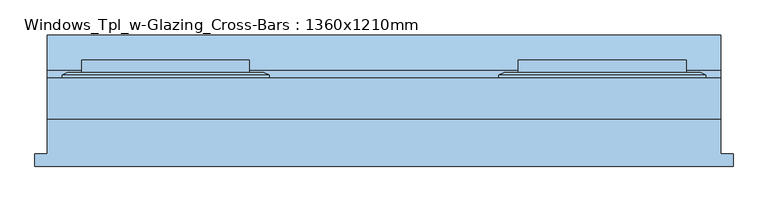
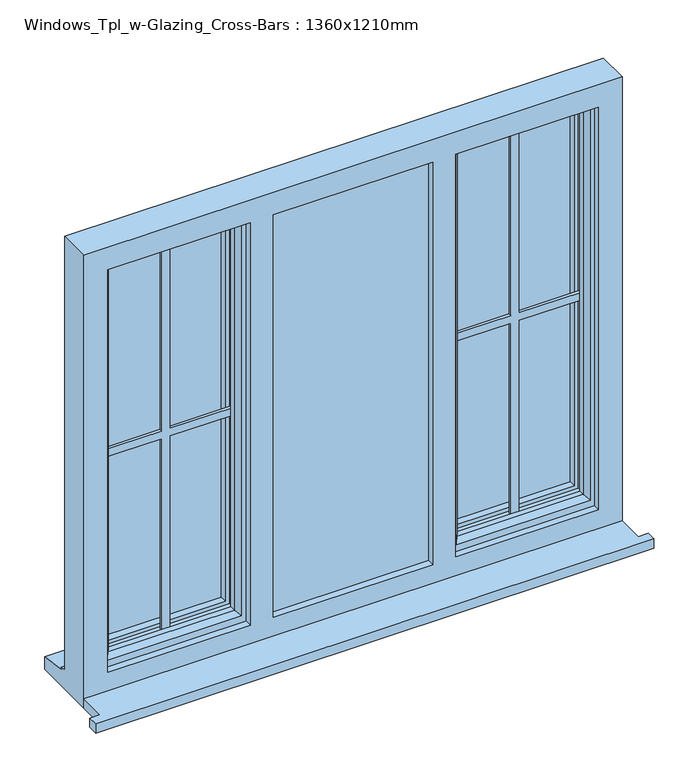
"""IFC4 building model written with IfcOpenShell, lengths in millimetres: window geometry, Windows_Tpl_w-Glazing_Cross-Bars : 1360x1210mm."""

from ifc_helpers import new_model, si_unit, frame, origin, place, context, project, spatial, polyline, outline, extrude, faceted_brep, source, transform, mapped, element, save


def windows_tpl_w_glazing_cross_bars_1360x1210mm_0306471f(model_context):
    return source(origin(), model_context, "Body", "SolidModel", [
        extrude(outline(polyline([(-1206.6666667, -118.1434322), (-1206.6666667, -93.1434322), (-1181.6666667, -93.1434322), (-1181.6666667, -22.9434322), (178.3333333, -22.9434322), (178.3333333, -93.1434322), (203.3333333, -93.1434322), (203.3333333, -118.1434322), (-1206.6666667, -118.1434322)])), frame((0.0, 0.0, 900.0), z_axis=(0.0, 0.0, 1.0), x_axis=(1.0, 0.0, 0.0)), (0.0, 0.0, 1.0), 25.0),
        faceted_brep([(-270.0, 60.0565678, 2080.0), (-270.0, 65.8300705, 2080.0), (-270.0, 65.8300705, 953.0), (-270.0, 60.0565678, 953.0), (-260.0, -4.9434322, 2070.0), (-260.0, 60.0565678, 2070.0), (-260.0, 60.0565678, 963.0), (-260.0, -4.9434322, 963.0), (-220.0, 9.5494677, 2030.0), (-230.1480377, -4.9434322, 2040.1480377), (-230.1480377, -4.9434322, 992.8519623), (-220.0, 9.5494677, 1003.0), (-220.0, 24.0565678, 2030.0), (-220.0, 24.0565678, 1003.0), (-230.0, 48.0565678, 2040.0), (-230.0, 24.0565678, 2040.0), (-230.0, 24.0565678, 993.0), (-230.0, 48.0565678, 993.0), (-220.0, 65.8300705, 2030.0), (-220.0, 48.0565678, 2030.0), (-220.0, 48.0565678, 1003.0), (-220.0, 65.8300705, 1003.0), (-237.4457548, 71.6035732, 2047.4457548), (-237.4457548, 71.6035732, 985.5542452), (-259.2153903, 71.6035732, 2069.2153903), (-259.2153903, 71.6035732, 963.7846097), (148.3333333, 65.8300705, 953.0), (148.3333333, 60.0565678, 953.0), (138.3333333, 60.0565678, 963.0), (138.3333333, -4.9434322, 963.0), (108.4813711, -4.9434322, 992.8519623), (98.3333333, 9.5494677, 1003.0), (98.3333333, 24.0565678, 1003.0), (108.3333333, 24.0565678, 993.0), (108.3333333, 48.0565678, 993.0), (98.3333333, 48.0565678, 1003.0), (98.3333333, 65.8300705, 1003.0), (115.7790881, 71.6035732, 985.5542452), (137.5487236, 71.6035732, 963.7846097), (148.3333333, 65.8300705, 2080.0), (148.3333333, 60.0565678, 2080.0), (138.3333333, 60.0565678, 2070.0), (138.3333333, -4.9434322, 2070.0), (108.4813711, -4.9434322, 2040.1480377), (98.3333333, 9.5494677, 2030.0), (98.3333333, 24.0565678, 2030.0), (108.3333333, 24.0565678, 2040.0), (108.3333333, 48.0565678, 2040.0), (98.3333333, 48.0565678, 2030.0), (98.3333333, 65.8300705, 2030.0), (115.7790881, 71.6035732, 2047.4457548), (137.5487236, 71.6035732, 2069.2153903)], [[[0, 1, 2, 3]], [[4, 5, 6, 7]], [[8, 9, 10, 11]], [[12, 8, 11, 13]], [[14, 15, 16, 17]], [[18, 19, 20, 21]], [[22, 18, 21, 23]], [[1, 24, 25, 2]], [[3, 2, 26, 27]], [[7, 6, 28, 29]], [[11, 10, 30, 31]], [[13, 11, 31, 32]], [[17, 16, 33, 34]], [[21, 20, 35, 36]], [[23, 21, 36, 37]], [[2, 25, 38, 26]], [[27, 26, 39, 40]], [[29, 28, 41, 42]], [[31, 30, 43, 44]], [[32, 31, 44, 45]], [[34, 33, 46, 47]], [[36, 35, 48, 49]], [[37, 36, 49, 50]], [[26, 38, 51, 39]], [[40, 39, 1, 0]], [[3, 27, 40, 0], [5, 41, 28, 6]], [[42, 41, 5, 4]], [[7, 29, 42, 4], [9, 43, 30, 10]], [[44, 43, 9, 8]], [[45, 44, 8, 12]], [[15, 46, 33, 16], [13, 32, 45, 12]], [[47, 46, 15, 14]], [[17, 34, 47, 14], [19, 48, 35, 20]], [[49, 48, 19, 18]], [[50, 49, 18, 22]], [[24, 51, 38, 25], [23, 37, 50, 22]], [[39, 51, 24, 1]]]),
        faceted_brep([(-733.3333333, 60.0565678, 2080.0), (-733.3333333, 65.8300705, 2080.0), (-1151.6666667, 65.8300705, 2080.0), (-1151.6666667, 60.0565678, 2080.0), (-743.3333333, -4.9434322, 2070.0), (-743.3333333, 60.0565678, 2070.0), (-1141.6666667, 60.0565678, 2070.0), (-1141.6666667, -4.9434322, 2070.0), (-783.3333333, 9.5494677, 2030.0), (-773.1852956, -4.9434322, 2040.1480377), (-1111.8147044, -4.9434322, 2040.1480377), (-1101.6666667, 9.5494677, 2030.0), (-783.3333333, 24.0565678, 2030.0), (-1101.6666667, 24.0565678, 2030.0), (-773.3333333, 48.0565678, 2040.0), (-773.3333333, 24.0565678, 2040.0), (-1111.6666667, 24.0565678, 2040.0), (-1111.6666667, 48.0565678, 2040.0), (-783.3333333, 65.8300705, 2030.0), (-783.3333333, 48.0565678, 2030.0), (-1101.6666667, 48.0565678, 2030.0), (-1101.6666667, 65.8300705, 2030.0), (-765.8875785, 71.6035732, 2047.4457548), (-1119.1124215, 71.6035732, 2047.4457548), (-744.117943, 71.6035732, 2069.2153903), (-1140.882057, 71.6035732, 2069.2153903), (-1151.6666667, 65.8300705, 953.0), (-1151.6666667, 60.0565678, 953.0), (-1141.6666667, 60.0565678, 963.0), (-1141.6666667, -4.9434322, 963.0), (-1111.8147044, -4.9434322, 992.8519623), (-1101.6666667, 9.5494677, 1003.0), (-1101.6666667, 24.0565678, 1003.0), (-1111.6666667, 24.0565678, 993.0), (-1111.6666667, 48.0565678, 993.0), (-1101.6666667, 48.0565678, 1003.0), (-1101.6666667, 65.8300705, 1003.0), (-1119.1124215, 71.6035732, 985.5542452), (-1140.882057, 71.6035732, 963.7846097), (-733.3333333, 65.8300705, 953.0), (-733.3333333, 60.0565678, 953.0), (-743.3333333, 60.0565678, 963.0), (-743.3333333, -4.9434322, 963.0), (-773.1852956, -4.9434322, 992.8519623), (-783.3333333, 9.5494677, 1003.0), (-783.3333333, 24.0565678, 1003.0), (-773.3333333, 24.0565678, 993.0), (-773.3333333, 48.0565678, 993.0), (-783.3333333, 48.0565678, 1003.0), (-783.3333333, 65.8300705, 1003.0), (-765.8875785, 71.6035732, 985.5542452), (-744.117943, 71.6035732, 963.7846097)], [[[0, 1, 2, 3]], [[4, 5, 6, 7]], [[8, 9, 10, 11]], [[12, 8, 11, 13]], [[14, 15, 16, 17]], [[18, 19, 20, 21]], [[22, 18, 21, 23]], [[1, 24, 25, 2]], [[3, 2, 26, 27]], [[7, 6, 28, 29]], [[11, 10, 30, 31]], [[13, 11, 31, 32]], [[17, 16, 33, 34]], [[21, 20, 35, 36]], [[23, 21, 36, 37]], [[2, 25, 38, 26]], [[27, 26, 39, 40]], [[0, 3, 27, 40], [41, 28, 6, 5]], [[29, 28, 41, 42]], [[4, 7, 29, 42], [43, 30, 10, 9]], [[31, 30, 43, 44]], [[32, 31, 44, 45]], [[46, 33, 16, 15], [12, 13, 32, 45]], [[34, 33, 46, 47]], [[14, 17, 34, 47], [48, 35, 20, 19]], [[36, 35, 48, 49]], [[37, 36, 49, 50]], [[51, 38, 25, 24], [22, 23, 37, 50]], [[26, 38, 51, 39]], [[40, 39, 1, 0]], [[42, 41, 5, 4]], [[44, 43, 9, 8]], [[45, 44, 8, 12]], [[47, 46, 15, 14]], [[49, 48, 19, 18]], [[50, 49, 18, 22]], [[39, 51, 24, 1]]]),
        extrude(outline(polyline([(993.0, -70.8333333), (993.0, -50.8333333), (1506.5, -50.8333333), (1506.5, 108.3333333), (1526.5, 108.3333333), (1526.5, -50.8333333), (2040.1480377, -50.8333333), (2040.1480377, -70.8333333), (1526.5, -70.8333333), (1526.5, -230.1480377), (1506.5, -230.1480377), (1506.5, -70.8333333), (993.0, -70.8333333)])), frame((0.0, 32.0565678, 0.0), z_axis=(0.0, 1.0, 0.0), x_axis=(0.0, 0.0, 1.0)), (0.0, 0.0, 1.0), 8.0),
        extrude(outline(polyline([(993.0, -952.5), (993.0, -932.5), (1506.5, -932.5), (1506.5, -773.3333333), (1526.5, -773.3333333), (1526.5, -932.5), (2040.1480377, -932.5), (2040.1480377, -952.5), (1526.5, -952.5), (1526.5, -1111.6666667), (1506.5, -1111.6666667), (1506.5, -952.5), (993.0, -952.5)])), frame((0.0, 32.0565678, 0.0), z_axis=(0.0, 1.0, 0.0), x_axis=(0.0, 0.0, 1.0)), (0.0, 0.0, 1.0), 8.0),
        extrude(outline(polyline([(963.0, -511.6666667), (963.0, -491.6666667), (1506.5, -491.6666667), (1506.5, -290.0), (1526.5, -290.0), (1526.5, -491.6666667), (2070.0, -491.6666667), (2070.0, -511.6666667), (1526.5, -511.6666667), (1526.5, -713.3333333), (1506.5, -713.3333333), (1506.5, -511.6666667), (963.0, -511.6666667)])), frame((0.0, 3.0565678, 0.0), z_axis=(0.0, 1.0, 0.0), x_axis=(0.0, 0.0, 1.0)), (0.0, 0.0, 1.0), 8.0),
        faceted_brep([(178.3333333, -22.9434322, 2110.0), (-1181.6666667, -22.9434322, 2110.0), (-1181.6666667, -22.9434322, 900.0), (178.3333333, -22.9434322, 900.0), (118.3333333, -22.9434322, 2050.0), (118.3333333, -22.9434322, 975.0), (-242.0, -22.9434322, 975.0), (-242.0, -22.9434322, 2050.0), (-300.0, -22.9434322, 2050.0), (-300.0, -22.9434322, 975.0), (-703.3333333, -22.9434322, 975.0), (-703.3333333, -22.9434322, 2050.0), (-761.3333333, -22.9434322, 2050.0), (-761.3333333, -22.9434322, 975.0), (-1121.6666667, -22.9434322, 975.0), (-1121.6666667, -22.9434322, 2050.0), (-1181.6666667, 60.0565678, 2110.0), (-1181.6666667, 60.0565678, 951.0), (-1181.6666667, 75.0565678, 949.68767), (-1181.6666667, 75.0565678, 944.7449676), (-1181.6666667, 147.5565678, 933.8088847), (-1181.6666667, 147.5565678, 900.0), (178.3333333, 60.0565678, 2110.0), (178.3333333, 60.0565678, 951.0), (-1141.6666667, 60.0565678, 2070.0), (-1141.6666667, 60.0565678, 963.0), (-743.3333333, 60.0565678, 963.0), (-743.3333333, 60.0565678, 2070.0), (-703.3333333, 60.0565678, 2070.0), (-703.3333333, 60.0565678, 963.0), (-300.0, 60.0565678, 963.0), (-300.0, 60.0565678, 2070.0), (-260.0, 60.0565678, 2070.0), (-260.0, 60.0565678, 963.0), (138.3333333, 60.0565678, 963.0), (138.3333333, 60.0565678, 2070.0), (-1141.6666667, -4.9434322, 2070.0), (-1141.6666667, -4.9434322, 963.0), (-713.3333333, -4.9434322, 2070.0), (-290.0, -4.9434322, 2070.0), (-290.0, -4.9434322, 963.0), (-713.3333333, -4.9434322, 963.0), (-300.0, -4.9434322, 2050.0), (-703.3333333, -4.9434322, 2050.0), (-703.3333333, -4.9434322, 975.0), (-300.0, -4.9434322, 975.0), (-260.0, -4.9434322, 2070.0), (138.3333333, -4.9434322, 2070.0), (138.3333333, -4.9434322, 963.0), (-260.0, -4.9434322, 963.0), (118.3333333, -4.9434322, 2050.0), (-242.0, -4.9434322, 2050.0), (-242.0, -4.9434322, 975.0), (118.3333333, -4.9434322, 975.0), (-743.3333333, -4.9434322, 2070.0), (-743.3333333, -4.9434322, 963.0), (-761.3333333, -4.9434322, 2050.0), (-1121.6666667, -4.9434322, 2050.0), (-1121.6666667, -4.9434322, 975.0), (-761.3333333, -4.9434322, 975.0), (-703.3333333, 19.0565678, 2070.0), (-300.0, 19.0565678, 2070.0), (-290.0, 19.0565678, 2070.0), (-713.3333333, 19.0565678, 2070.0), (178.3333333, 147.5565678, 900.0), (178.3333333, 147.5565678, 933.8088847), (178.3333333, 75.0565678, 944.7449676), (178.3333333, 75.0565678, 949.68767), (-703.3333333, 19.0565678, 963.0), (-713.3333333, 19.0565678, 963.0), (-290.0, 19.0565678, 963.0), (-300.0, 19.0565678, 963.0)], [[[0, 1, 2, 3], [4, 5, 6, 7], [8, 9, 10, 11], [12, 13, 14, 15]], [[2, 1, 16, 17, 18, 19, 20, 21]], [[17, 16, 22, 23], [24, 25, 26, 27], [28, 29, 30, 31], [32, 33, 34, 35]], [[25, 24, 36, 37]], [[38, 39, 40, 41], [42, 43, 44, 45]], [[46, 47, 48, 49], [50, 51, 52, 53]], [[36, 54, 55, 37], [56, 57, 58, 59]], [[57, 15, 14, 58]], [[1, 0, 22, 16]], [[36, 24, 27, 54]], [[35, 47, 46, 32]], [[60, 28, 31, 61, 62, 39, 38, 63]], [[15, 57, 56, 12]], [[50, 4, 7, 51]], [[11, 43, 42, 8]], [[23, 22, 0, 3, 64, 65, 66, 67]], [[35, 34, 48, 47]], [[4, 50, 53, 5]], [[43, 11, 10, 44]], [[12, 56, 59, 13]], [[27, 26, 55, 54]], [[29, 28, 60, 68]], [[68, 60, 63, 69]], [[69, 63, 38, 41]], [[62, 70, 40, 39]], [[70, 62, 61, 71]], [[71, 61, 31, 30]], [[33, 32, 46, 49]], [[51, 7, 6, 52]], [[8, 42, 45, 9]], [[64, 3, 2, 21]], [[65, 64, 21, 20]], [[66, 65, 20, 19]], [[67, 66, 19, 18]], [[23, 67, 18, 17]], [[26, 25, 37, 55]], [[34, 33, 49, 48]], [[41, 40, 70, 71, 30, 29, 68, 69]], [[6, 5, 53, 52]], [[45, 44, 10, 9]], [[59, 58, 14, 13]]]),
        extrude(outline(polyline([(-713.3333333, 19.0565678), (-290.0, 19.0565678), (-290.0, -4.9434322), (-713.3333333, -4.9434322), (-713.3333333, 19.0565678)])), frame((0.0, 0.0, 963.0), z_axis=(0.0, 0.0, 1.0), x_axis=(1.0, 0.0, 0.0)), (0.0, 0.0, 1.0), 1107.0),
        extrude(outline(polyline([(-773.3333333, 72.4565678), (-1111.6666667, 72.4565678), (-1111.6666667, 96.4565678), (-773.3333333, 96.4565678), (-773.3333333, 72.4565678)])), frame((0.0, 0.0, 993.0), z_axis=(0.0, 0.0, 1.0), x_axis=(1.0, 0.0, 0.0)), (0.0, 0.0, 1.0), 1047.0),
        extrude(outline(polyline([(108.4813711, 72.4565678), (-230.1480377, 72.4565678), (-230.1480377, 96.4565678), (108.4813711, 96.4565678), (108.4813711, 72.4565678)])), frame((0.0, 0.0, 992.8519623), z_axis=(0.0, 0.0, 1.0), x_axis=(1.0, 0.0, 0.0)), (0.0, 0.0, 1.0), 1047.2960754),
    ])


if __name__ == "__main__":
    model = new_model("IFC4")
    model_context = context("Model", 3, world=origin())
    ifc_project = project(units=[si_unit("LENGTHUNIT", "METRE", prefix="MILLI")], contexts=[model_context])
    site = spatial("IfcSite", under=ifc_project)
    building = spatial("IfcBuilding", under=site)
    placement = place(None, origin())
    windows_tpl_w_glazing_cross_bars_1360x1210mm_shape = windows_tpl_w_glazing_cross_bars_1360x1210mm_0306471f(model_context)
    element("IfcWindow", 1, ObjectType="Windows_Tpl_w-Glazing_Cross-Bars : 1360x1210mm", at=placement, inside=building, context=model_context, shape_type="MappedRepresentation", body=[
        mapped(windows_tpl_w_glazing_cross_bars_1360x1210mm_shape, transform((0.0, 0.0, 0.0), x_axis=(1.0, 0.0, 0.0), y_axis=(0.0, 1.0, 0.0), z_axis=(0.0, 0.0, 1.0))),
    ])
    save(model, "model.ifc")

# Revit data of these elements
# Type "Windows_Tpl_w-Glazing_Cross-Bars : 1360x1210mm"
#   Type Mark = "21"
#   Operation = "TriplePanelVertical"
#   Construction Type Id = "GSP4R"
#   Manufacturer = "Revit"
#   Keynote = "L10"
#   Analytic Construction = "1/8 in Pilkington single glazing"
#   Wrap Layers (Ext) from Ext = 0' - 4.03543"
#   Wrap Layers (Int) from Ext = 0' - 6.98819"
#   Window Board Projection = 0' - 0.98425"
#   Window Board Extension = 0' - 0.98425"
#   Visual Light Transmittance = 0.9
#   Solar Heat Gain Coefficient = 0.78
#   Rough Width = 4' - 5.54331"
#   Rough Height = 3' - 11.6378"
#   Height = 3' - 11.6378"
#   Width = 4' - 5.54331"
#   Heat Transfer Coefficient (U) = 0.6496 BTU/(h·ft²·°F)
#   Glazing Thickness = 0' - 0.94488"
#   Glazing Bar Thickness = 0' - 0.7874"
#   FrameOffset - External = 0' - 1.9685"
#   Frame Depth = 0' - 2.55906"
#   Default Head Height = 6' - 11.07087"
#   Cill Depth = 0' - 3.44488"
#   Cavity Closer Width = 0' - 1.9685"
#   Cavity Closer Offset from Ext = 0' - 4.03543"
#   Cavity Closer Depth = 0' - 3.34646"
#   Vis - Glazing Bars = yes
#   Vis - Cavity Closers = yes
#   Define Thermal Properties by = 1
#   Material Trim = Window Frame
#   Material Glazing Bars = Window Frame
#   Material Glass = Glass
#   Material Frame = Window Frame
#   Wall Closure = (empty or 0)
# Element 1 (IfcWindow, "Windows_Tpl_w-Glazing_Cross-Bars : 1360x1210mm")
#   Materials on its faces: "Window Frame", "Glass"
# Materials
#   "Window Frame": colour RGB 249 249 249, transparency 0
#   "Glass": class "Glass", colour RGB 0 128 192, transparency 0.75, Description = "Soda Lime Glass", Cost = 0
